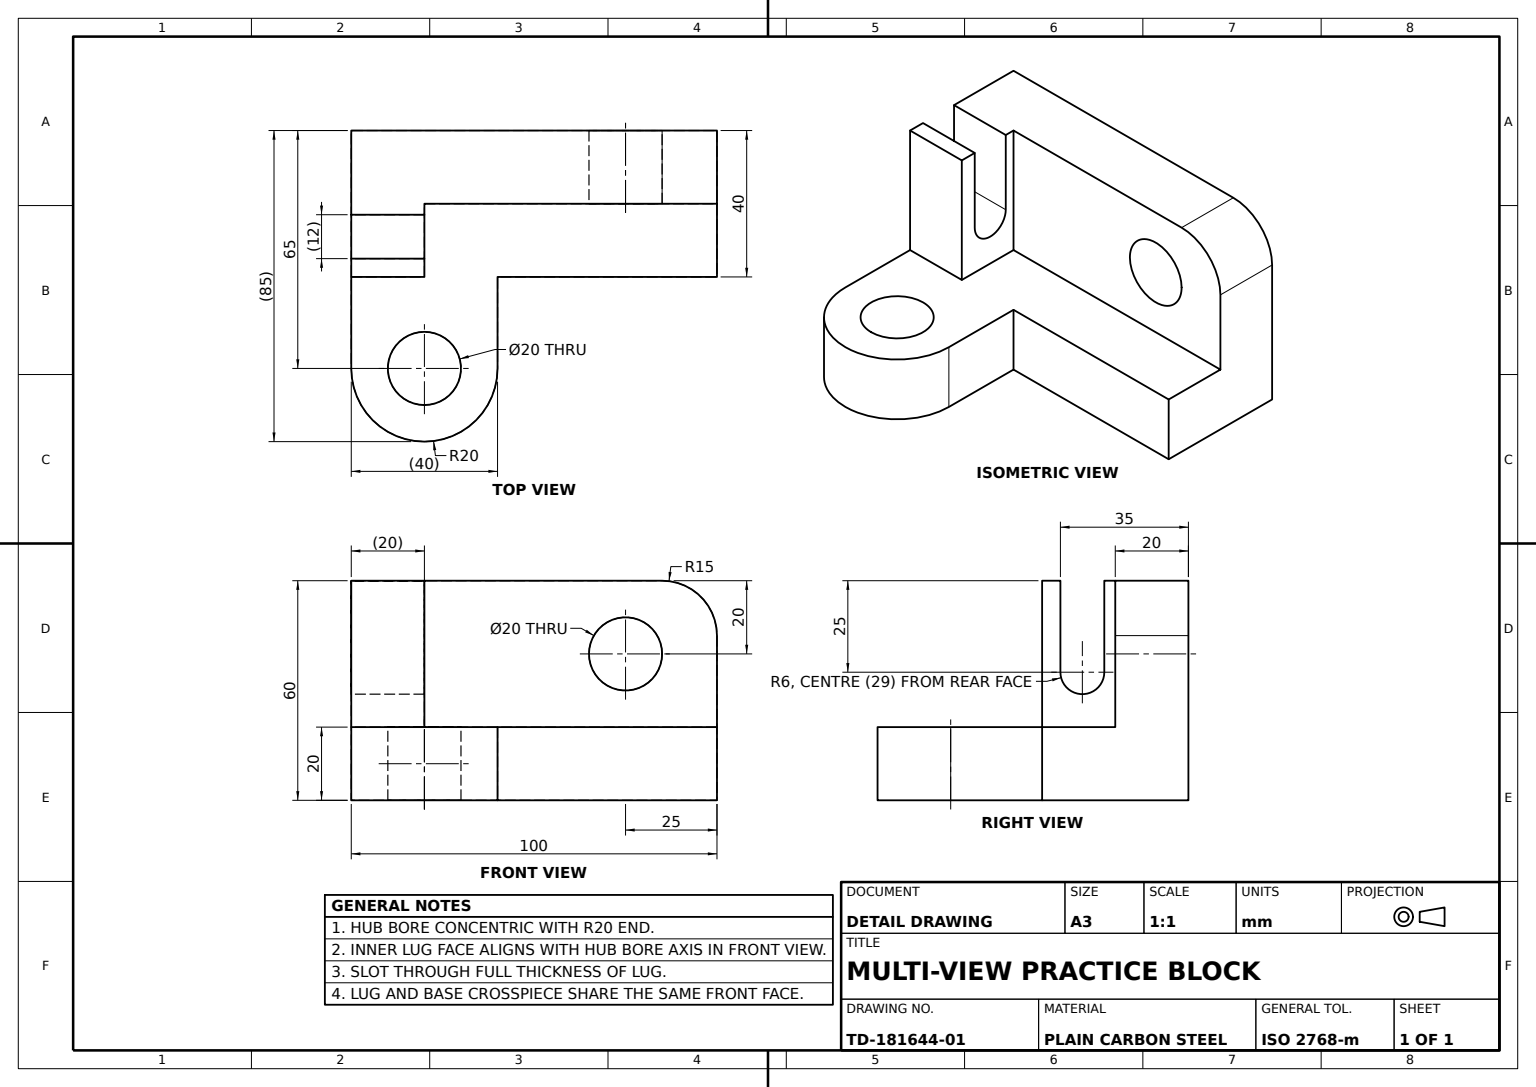
from build123d import *

# Parameters (mm, degrees)
BASE_BLOCK_DEPTH   = 20
HUB_BOSS_DEPTH     = 20
LEG_PROFILE_W      = 60
LEG_PROFILE_H      = 20
LEG_DEPTH          = 20
TOP_ARM_DEPTH      = 20
HUB_BORE_SKETCH_R  = 10
HUB_BORE_CUT_DEPTH = 20
LEG_SLOT_SKETCH_R  = 10
LEG_SLOT_CUT_DEPTH = 20


with BuildPart() as part:
    # Base Block Profile → Base Block (new body)
    with BuildSketch(Plane.XY):
        with BuildLine():
            Line((0, 0), (-85, 0))
            ThreePointArc((-85, 0), (-95.606601718, 4.393398282), (-100, 15))
            Line((-100, 15), (-100, 60))
            Line((-100, 60), (0, 60))
            Line((0, 60), (0, 0))
        make_face()
    extrude(amount=BASE_BLOCK_DEPTH)

    # Hub Boss Profile → Hub Boss (add)
    with BuildSketch(Plane(origin=(0, 0, 0), x_dir=(0, 0, -1), z_dir=(1, 0, 0))):
        with BuildLine():
            Line((-20, 0), (-20, 40))
            Line((-20, 40), (-40, 40))
            Line((-40, 40), (-40, 0))
            Line((-40, 0), (-35, 0))
            Line((-35, 0), (-35, 25))
            ThreePointArc((-35, 25), (-29, 31), (-23, 25))
            Line((-23, 25), (-23, 0))
            Line((-23, 0), (-20, 0))
        make_face()
    extrude(amount=-HUB_BOSS_DEPTH)

    # Leg Profile → Leg (add)
    with BuildSketch(Plane(origin=(0, 60, 0), x_dir=(1, 0, 0), z_dir=(0, 1, 0))):
        with Locations((-70, -30)):
            Rectangle(LEG_PROFILE_W, LEG_PROFILE_H)
    extrude(amount=-LEG_DEPTH)

    # Top Arm Profile → Top Arm (add)
    with BuildSketch(Plane(origin=(0, 60, 0), x_dir=(1, 0, 0), z_dir=(0, 1, 0))):
        with BuildLine():
            Line((-40, -20), (0, -20))
            Line((0, -20), (0, -65))
            ThreePointArc((0, -65), (-20, -85), (-40, -65))
            Line((-40, -65), (-40, -20))
        make_face()
    extrude(amount=-TOP_ARM_DEPTH)

    # Hub Bore Sketch → Hub Bore Cut (cut)
    with BuildSketch(Plane.XZ.offset(-40)):
        with Locations(Location((-20, 65, 0), (0, 0, 270))):
            Circle(HUB_BORE_SKETCH_R)
    extrude(amount=-HUB_BORE_CUT_DEPTH, mode=Mode.SUBTRACT)

    # Leg Slot Sketch → Leg Slot Cut (cut)
    with BuildSketch(Plane.XY.offset(20)):
        with Locations((-75, 20)):
            Circle(LEG_SLOT_SKETCH_R)
    extrude(amount=-LEG_SLOT_CUT_DEPTH, mode=Mode.SUBTRACT)


solid = part.part
